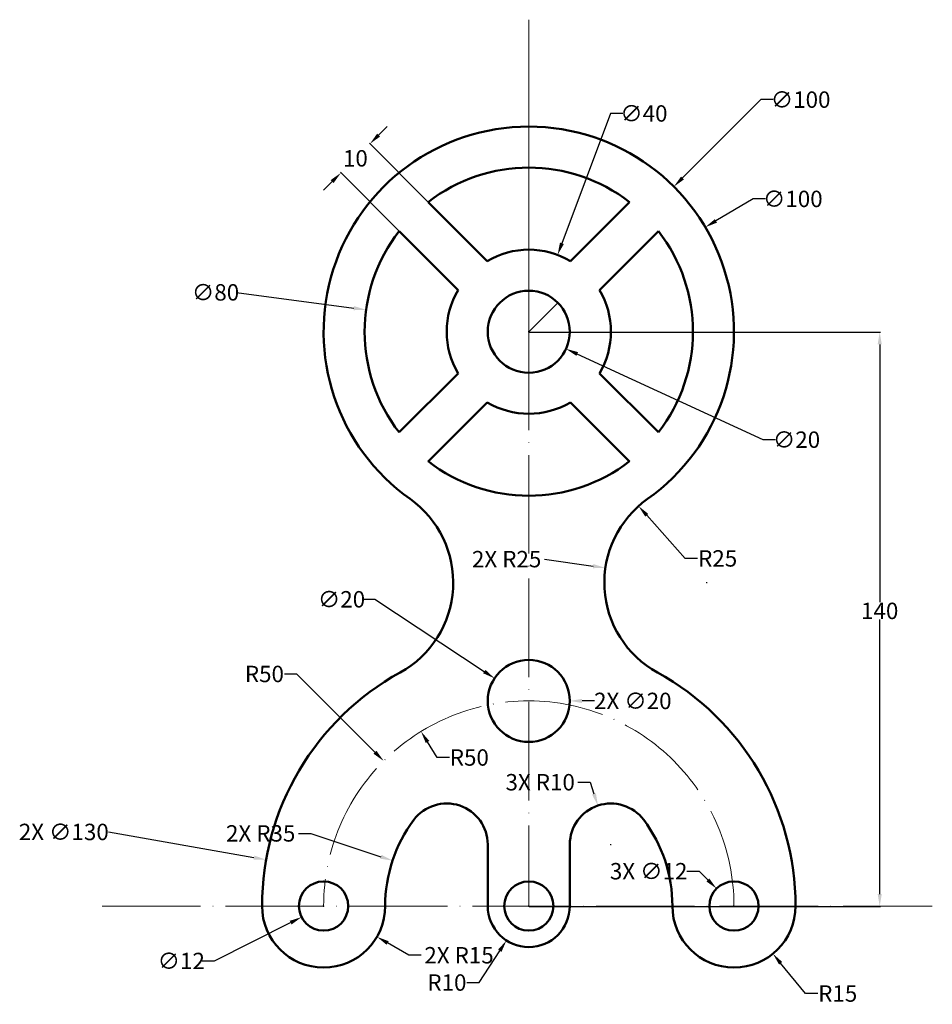
# Model space of a CAD drawing. Units: inches. Extents: x 540 to 763, y 295 to 535.
import ezdxf

# ---------------------------------------------------------------- set-up
doc = ezdxf.new("R2010")
doc.units = ezdxf.units.IN
doc.header["$MEASUREMENT"] = 0
doc.linetypes.add('ACAD_ISO04W100', pattern=[30, 24, -3, 0, -3])
for name, color, linetype, lineweight in [('M-CNTR', 4, 'ACAD_ISO04W100', 18), ('M-CONS', 8, 'Continuous', 13), ('M-DIMS', 2, 'Continuous', 25), ('M-OUTL', 7, 'Continuous', 50)]:
    doc.layers.add(name, color=color, linetype=linetype, lineweight=lineweight)
doc.styles.get("Standard").update_dxf_attribs({"font": 'arial.ttf'})
doc.dimstyles.get("Standard").update_dxf_attribs({"dimtxt": 4, "dimasz": 3, "dimexe": 0.18, "dimexo": 0.0625, "dimgap": 0.09, "dimtad": 0, "dimtih": 1, "dimtoh": 1, "dimdec": 0, "dimzin": 0, "dimdsep": 46, "dimtxsty": 'Standard', "dimcen": 0.09, "dimadec": 0, "dimazin": 0, "dimtfac": 1, "dimtdec": 0, "dimtofl": 0, "dimtmove": 0, "dimatfit": 3, "dimfxl": 1, "dimtolj": 1, "dimtzin": 0, "dimarcsym": 0})

# ---------------------------------------------------------------- blocks, each defined once
blk = doc.blocks.new('*U1')
for p, q in [((-10.72, -3.65), (3.65, 10.72)), ((-3.65, -10.72), (10.72, 3.65))]:
    blk.add_line(p, q)
blk = doc.blocks.new('*U2')
at = {"layer": 'M-OUTL', "color": 0, "linetype": 'ByBlock', "lineweight": -2, "transparency": 16777216}
for p, rotation in [((643.5, 480.1), 90.00000000000003), ((643.5, 438.34), 180), ((685.26, 438.34), 270.0000000000001)]:
    blk.add_blockref('*U1', p, dxfattribs=dict(at, rotation=rotation))
blk.add_blockref('*U1', (685.26, 480.1), dxfattribs=at)
blk = doc.blocks.new('*D3')
at = {"layer": 'Defpoints', "color": 0, "transparency": 16777216}
for p in [(625.66, 505.02), (639.85, 490.82), (632.78, 483.75)]:
    blk.add_point(p, dxfattribs=at)
at = {"layer": 'M-DIMS', "color": 0, "lineweight": -2, "transparency": 16777216}
for p, q in [((627.78, 507.14), (629.9, 509.26)), ((639.81, 490.86), (625.53, 505.14)), ((632.74, 483.79), (618.46, 498.07)), ((616.46, 495.82), (614.34, 493.7))]:
    blk.add_line(p, q, dxfattribs=at)
at = {"layer": 'M-DIMS', "color": 0, "transparency": 16777216}
for points in [[(627.42, 507.49), (628.13, 506.78), (625.66, 505.02)], [(616.11, 496.18), (616.82, 495.47), (618.59, 497.94)]]:
    blk.add_solid(points, dxfattribs=at)
at = {"layer": 'M-DIMS', "color": 0, "transparency": 16777216, "insert": (622.12, 501.48), "char_height": 4, "attachment_point": 5}
blk.add_mtext('\\A1;10', dxfattribs=at)
blk = doc.blocks.new('*D4')
at = {"layer": 'Defpoints', "color": 0, "transparency": 16777216}
for p in [(707.4, 484.7), (621.36, 433.74)]:
    blk.add_point(p, dxfattribs=at)
at = {"layer": 'M-DIMS', "color": 0, "lineweight": -2, "transparency": 16777216}
for p, q in [((719.05, 491.59), (709.98, 486.23)), ((722.05, 491.59), (719.05, 491.59)), ((664.29, 459.22), (664.47, 459.22)), ((664.38, 459.13), (664.38, 459.31))]:
    blk.add_line(p, q, dxfattribs=at)
at = {"layer": 'M-DIMS', "color": 0, "transparency": 16777216}
blk.add_solid([(709.73, 486.66), (710.24, 485.8), (707.4, 484.7)], dxfattribs=at)
at = {"layer": 'M-DIMS', "color": 0, "transparency": 16777216, "insert": (728.72, 491.59), "char_height": 4, "attachment_point": 5}
blk.add_mtext('\\A1;∅100', dxfattribs=at)
blk = doc.blocks.new('*D5')
at = {"layer": 'Defpoints', "color": 0, "transparency": 16777216}
for p in [(624.74, 464.56), (704.02, 453.88)]:
    blk.add_point(p, dxfattribs=at)
at = {"layer": 'M-DIMS', "color": 0, "lineweight": -2, "transparency": 16777216}
for p, q in [((593.17, 468.81), (621.76, 464.96)), ((664.29, 459.22), (664.47, 459.22)), ((664.38, 459.13), (664.38, 459.31))]:
    blk.add_line(p, q, dxfattribs=at)
at = {"layer": 'M-DIMS', "color": 0, "transparency": 16777216}
blk.add_solid([(621.83, 465.45), (621.7, 464.46), (624.74, 464.56)], dxfattribs=at)
at = {"layer": 'M-DIMS', "color": 0, "transparency": 16777216, "insert": (588.04, 468.81), "char_height": 4, "attachment_point": 5}
blk.add_mtext('\\A1;∅80', dxfattribs=at)
blk = doc.blocks.new('*D6')
at = {"layer": 'Defpoints', "color": 0, "transparency": 16777216}
for p in [(671.4, 477.95), (657.36, 440.49)]:
    blk.add_point(p, dxfattribs=at)
at = {"layer": 'M-DIMS', "color": 0, "lineweight": -2, "transparency": 16777216}
for p, q in [((684.31, 512.42), (672.45, 480.76)), ((687.31, 512.42), (684.31, 512.42)), ((664.29, 459.22), (664.47, 459.22)), ((664.38, 459.13), (664.38, 459.31))]:
    blk.add_line(p, q, dxfattribs=at)
at = {"layer": 'M-DIMS', "color": 0, "transparency": 16777216}
blk.add_solid([(671.98, 480.94), (672.92, 480.58), (671.4, 477.95)], dxfattribs=at)
at = {"layer": 'M-DIMS', "color": 0, "transparency": 16777216, "insert": (692.43, 512.42), "char_height": 4, "attachment_point": 5}
blk.add_mtext('\\A1;∅40', dxfattribs=at)
blk = doc.blocks.new('*D7')
at = {"layer": 'Defpoints', "color": 0, "transparency": 16777216}
for p in [(655.3, 463.41), (673.46, 455.04)]:
    blk.add_point(p, dxfattribs=at)
at = {"layer": 'M-DIMS', "color": 0, "lineweight": -2, "transparency": 16777216}
for p, q in [((664.29, 459.22), (664.47, 459.22)), ((664.38, 459.13), (664.38, 459.31)), ((721.51, 432.9), (676.19, 453.78)), ((724.51, 432.9), (721.51, 432.9))]:
    blk.add_line(p, q, dxfattribs=at)
at = {"layer": 'M-DIMS', "color": 0, "transparency": 16777216}
blk.add_solid([(676.4, 454.24), (675.98, 453.33), (673.46, 455.04)], dxfattribs=at)
at = {"layer": 'M-DIMS', "color": 0, "transparency": 16777216, "insert": (729.63, 432.9), "char_height": 4, "attachment_point": 5}
blk.add_mtext('\\A1;∅20', dxfattribs=at)
blk = doc.blocks.new('*D8')
at = {"layer": 'Defpoints', "color": 0, "transparency": 16777216}
for p in [(664.38, 319.22), (658.94, 310.83)]:
    blk.add_point(p, dxfattribs=at)
at = {"layer": 'M-DIMS', "color": 0, "lineweight": -2, "transparency": 16777216}
for p, q in [((664.29, 319.22), (664.47, 319.22)), ((664.38, 319.13), (664.38, 319.31)), ((652.29, 300.57), (657.31, 308.31)), ((649.29, 300.57), (652.29, 300.57))]:
    blk.add_line(p, q, dxfattribs=at)
at = {"layer": 'M-DIMS', "color": 0, "transparency": 16777216}
blk.add_solid([(656.89, 308.58), (657.73, 308.04), (658.94, 310.83)], dxfattribs=at)
at = {"layer": 'M-DIMS', "color": 0, "transparency": 16777216, "insert": (644.43, 300.57), "char_height": 4, "attachment_point": 5}
blk.add_mtext('\\A1;R10', dxfattribs=at)
blk = doc.blocks.new('*D9')
at = {"layer": 'Defpoints', "color": 0, "transparency": 16777216}
for p in [(619.74, 321.92), (609.02, 316.52)]:
    blk.add_point(p, dxfattribs=at)
at = {"layer": 'M-DIMS', "color": 0, "lineweight": -2, "transparency": 16777216}
for p, q in [((614.29, 319.22), (614.47, 319.22)), ((614.38, 319.13), (614.38, 319.31)), ((587.8, 305.83), (606.34, 315.17)), ((584.8, 305.83), (587.8, 305.83))]:
    blk.add_line(p, q, dxfattribs=at)
at = {"layer": 'M-DIMS', "color": 0, "transparency": 16777216}
blk.add_solid([(606.12, 315.62), (606.57, 314.73), (609.02, 316.52)], dxfattribs=at)
at = {"layer": 'M-DIMS', "color": 0, "transparency": 16777216, "insert": (579.68, 305.83), "char_height": 4, "attachment_point": 5}
blk.add_mtext('\\A1;∅12', dxfattribs=at)
blk = doc.blocks.new('*D10')
at = {"layer": 'Defpoints', "color": 0, "transparency": 16777216}
for p in [(714.38, 319.22), (723.86, 307.6)]:
    blk.add_point(p, dxfattribs=at)
at = {"layer": 'M-DIMS', "color": 0, "lineweight": -2, "transparency": 16777216}
for p, q in [((714.29, 319.22), (714.47, 319.22)), ((714.38, 319.13), (714.38, 319.31)), ((731.78, 297.89), (725.76, 305.27)), ((734.78, 297.89), (731.78, 297.89))]:
    blk.add_line(p, q, dxfattribs=at)
at = {"layer": 'M-DIMS', "color": 0, "transparency": 16777216}
blk.add_solid([(726.14, 305.59), (725.37, 304.96), (723.86, 307.6)], dxfattribs=at)
at = {"layer": 'M-DIMS', "color": 0, "transparency": 16777216, "insert": (739.67, 297.89), "char_height": 4, "attachment_point": 5}
blk.add_mtext('\\A1;R15', dxfattribs=at)
blk = doc.blocks.new('*D11')
at = {"layer": 'Defpoints', "color": 0, "transparency": 16777216}
for p in [(656.03, 374.73), (672.72, 363.71)]:
    blk.add_point(p, dxfattribs=at)
at = {"layer": 'M-DIMS', "color": 0, "lineweight": -2, "transparency": 16777216}
for p, q in [((623.86, 393.99), (626.86, 393.99)), ((626.86, 393.99), (653.53, 376.38)), ((664.29, 369.22), (664.47, 369.22)), ((664.38, 369.13), (664.38, 369.31))]:
    blk.add_line(p, q, dxfattribs=at)
at = {"layer": 'M-DIMS', "color": 0, "transparency": 16777216}
blk.add_solid([(653.81, 376.8), (653.25, 375.97), (656.03, 374.73)], dxfattribs=at)
at = {"layer": 'M-DIMS', "color": 0, "transparency": 16777216, "insert": (618.74, 393.99), "char_height": 4, "attachment_point": 5}
blk.add_mtext('\\A1;∅20', dxfattribs=at)
blk = doc.blocks.new('*D12')
at = {"layer": 'Defpoints', "color": 0, "transparency": 16777216}
for p in [(638.12, 361.77), (664.38, 319.22)]:
    blk.add_point(p, dxfattribs=at)
at = {"layer": 'M-DIMS', "color": 0, "lineweight": -2, "transparency": 16777216}
for p, q in [((642.03, 355.43), (639.69, 359.22)), ((645.03, 355.43), (642.03, 355.43))]:
    blk.add_line(p, q, dxfattribs=at)
at = {"layer": 'M-DIMS', "color": 0, "transparency": 16777216}
blk.add_solid([(640.12, 359.48), (639.27, 358.95), (638.12, 361.77)], dxfattribs=at)
at = {"layer": 'M-DIMS', "color": 0, "transparency": 16777216, "insert": (649.89, 355.43), "char_height": 4, "attachment_point": 5}
blk.add_mtext('\\A1;R50', dxfattribs=at)
blk = doc.blocks.new('*D13')
at = {"layer": 'Defpoints', "color": 0, "transparency": 16777216}
for p in [(691.13, 416.71), (707.79, 398.06)]:
    blk.add_point(p, dxfattribs=at)
at = {"layer": 'M-DIMS', "color": 0, "lineweight": -2, "transparency": 16777216}
for p, q in [((702.52, 403.96), (693.13, 414.47)), ((705.52, 403.96), (702.52, 403.96))]:
    blk.add_line(p, q, dxfattribs=at)
at = {"layer": 'M-DIMS', "color": 0, "transparency": 16777216}
blk.add_solid([(693.5, 414.8), (692.76, 414.13), (691.13, 416.71)], dxfattribs=at)
at = {"layer": 'M-DIMS', "color": 0, "transparency": 16777216, "insert": (710.41, 403.96), "char_height": 4, "attachment_point": 5}
blk.add_mtext('\\A1;R25', dxfattribs=at)
blk = doc.blocks.new('*D14')
at = {"layer": 'Defpoints', "color": 0, "transparency": 16777216}
for p in [(664.38, 459.13), (664.38, 319.13), (749.9, 319.13)]:
    blk.add_point(p, dxfattribs=at)
at = {"layer": 'M-DIMS', "color": 0, "lineweight": -2, "transparency": 16777216}
for p, q in [((664.44, 459.13), (750.08, 459.13)), ((749.9, 456.13), (749.9, 393.31)), ((749.9, 322.13), (749.9, 389.04)), ((664.44, 319.13), (750.08, 319.13))]:
    blk.add_line(p, q, dxfattribs=at)
at = {"layer": 'M-DIMS', "color": 0, "transparency": 16777216}
for points in [[(749.4, 456.13), (750.4, 456.13), (749.9, 459.13)], [(749.4, 322.13), (750.4, 322.13), (749.9, 319.13)]]:
    blk.add_solid(points, dxfattribs=at)
at = {"layer": 'M-DIMS', "color": 0, "transparency": 16777216, "insert": (749.9, 391.17), "char_height": 4, "attachment_point": 5}
blk.add_mtext('\\A1;140', dxfattribs=at)
blk = doc.blocks.new('MOUNT-HOLE-D12')
blk.add_circle((0, 0), 6)
blk = doc.blocks.new('BORE-D20')
blk.add_circle((0, 0), 10)
blk = doc.blocks.new('*D17')
at = {"layer": 'Defpoints', "color": 0, "transparency": 16777216}
for p in [(600.37, 330.51), (728.39, 307.93)]:
    blk.add_point(p, dxfattribs=at)
at = {"layer": 'M-DIMS', "color": 0, "lineweight": -2, "transparency": 16777216}
for p, q in [((561.96, 337.28), (597.41, 331.03)), ((664.29, 319.22), (664.47, 319.22)), ((664.38, 319.13), (664.38, 319.31))]:
    blk.add_line(p, q, dxfattribs=at)
at = {"layer": 'M-DIMS', "color": 0, "transparency": 16777216}
blk.add_solid([(597.5, 331.52), (597.33, 330.54), (600.37, 330.51)], dxfattribs=at)
at = {"layer": 'M-DIMS', "color": 0, "transparency": 16777216, "insert": (551.06, 337.28), "char_height": 4, "attachment_point": 5}
blk.add_mtext('\\A1;2X ∅130', dxfattribs=at)
blk = doc.blocks.new('*D18')
at = {"layer": 'Defpoints', "color": 0, "transparency": 16777216}
for p in [(631.18, 330.29), (664.38, 319.22)]:
    blk.add_point(p, dxfattribs=at)
at = {"layer": 'M-DIMS', "color": 0, "lineweight": -2, "transparency": 16777216}
for p, q in [((608.25, 336.93), (611.25, 336.93)), ((611.25, 336.93), (628.33, 331.24)), ((664.29, 319.22), (664.47, 319.22)), ((664.38, 319.13), (664.38, 319.31))]:
    blk.add_line(p, q, dxfattribs=at)
at = {"layer": 'M-DIMS', "color": 0, "transparency": 16777216}
blk.add_solid([(628.49, 331.71), (628.17, 330.76), (631.18, 330.29)], dxfattribs=at)
at = {"layer": 'M-DIMS', "color": 0, "transparency": 16777216, "insert": (599.04, 336.93), "char_height": 4, "attachment_point": 5}
blk.add_mtext('\\A1;2X R35', dxfattribs=at)
blk = doc.blocks.new('*D19')
at = {"layer": 'Defpoints', "color": 0, "transparency": 16777216}
for p in [(681.22, 343.71), (684.38, 334.22)]:
    blk.add_point(p, dxfattribs=at)
at = {"layer": 'M-DIMS', "color": 0, "lineweight": -2, "transparency": 16777216}
for p, q in [((676.32, 349.4), (679.32, 349.4)), ((679.32, 349.4), (680.27, 346.55)), ((684.29, 334.22), (684.47, 334.22)), ((684.38, 334.13), (684.38, 334.31))]:
    blk.add_line(p, q, dxfattribs=at)
at = {"layer": 'M-DIMS', "color": 0, "transparency": 16777216}
blk.add_solid([(680.74, 346.71), (679.79, 346.4), (681.22, 343.71)], dxfattribs=at)
at = {"layer": 'M-DIMS', "color": 0, "transparency": 16777216, "insert": (667.16, 349.4), "char_height": 4, "attachment_point": 5}
blk.add_mtext('\\A1;3X R10', dxfattribs=at)
blk = doc.blocks.new('*D20')
at = {"layer": 'Defpoints', "color": 0, "transparency": 16777216}
for p in [(654.38, 369.22), (674.38, 369.22)]:
    blk.add_point(p, dxfattribs=at)
at = {"layer": 'M-DIMS', "color": 0, "lineweight": -2, "transparency": 16777216}
for p, q in [((664.29, 369.22), (664.47, 369.22)), ((664.38, 369.13), (664.38, 369.31)), ((680.38, 369.22), (677.38, 369.22))]:
    blk.add_line(p, q, dxfattribs=at)
at = {"layer": 'M-DIMS', "color": 0, "transparency": 16777216}
blk.add_solid([(677.38, 369.72), (677.38, 368.72), (674.38, 369.22)], dxfattribs=at)
at = {"layer": 'M-DIMS', "color": 0, "transparency": 16777216, "insert": (689.73, 369.22), "char_height": 4, "attachment_point": 5}
blk.add_mtext('\\A1;2X ∅20', dxfattribs=at)
blk = doc.blocks.new('*D21')
at = {"layer": 'Defpoints', "color": 0, "transparency": 16777216}
for p in [(710.14, 323.46), (718.62, 314.98)]:
    blk.add_point(p, dxfattribs=at)
at = {"layer": 'M-DIMS', "color": 0, "lineweight": -2, "transparency": 16777216}
for p, q in [((702.89, 327.71), (705.89, 327.71)), ((705.89, 327.71), (708.02, 325.59)), ((714.29, 319.22), (714.47, 319.22)), ((714.38, 319.13), (714.38, 319.31))]:
    blk.add_line(p, q, dxfattribs=at)
at = {"layer": 'M-DIMS', "color": 0, "transparency": 16777216}
blk.add_solid([(708.37, 325.94), (707.66, 325.23), (710.14, 323.46)], dxfattribs=at)
at = {"layer": 'M-DIMS', "color": 0, "transparency": 16777216, "insert": (693.59, 327.71), "char_height": 4, "attachment_point": 5}
blk.add_mtext('\\A1;3X ∅12', dxfattribs=at)
blk = doc.blocks.new('*D22')
at = {"layer": 'Defpoints', "color": 0, "transparency": 16777216}
for p in [(699.73, 494.58), (629.02, 423.87)]:
    blk.add_point(p, dxfattribs=at)
at = {"layer": 'M-DIMS', "color": 0, "lineweight": -2, "transparency": 16777216}
for p, q in [((720.95, 515.79), (701.86, 496.7)), ((723.95, 515.79), (720.95, 515.79)), ((664.29, 459.22), (664.47, 459.22)), ((664.38, 459.13), (664.38, 459.31))]:
    blk.add_line(p, q, dxfattribs=at)
at = {"layer": 'M-DIMS', "color": 0, "transparency": 16777216}
blk.add_solid([(701.5, 497.05), (702.21, 496.35), (699.73, 494.58)], dxfattribs=at)
at = {"layer": 'M-DIMS', "color": 0, "transparency": 16777216, "insert": (730.63, 515.79), "char_height": 4, "attachment_point": 5}
blk.add_mtext('\\A1;∅100', dxfattribs=at)
blk = doc.blocks.new('*D23')
at = {"layer": 'Defpoints', "color": 0, "transparency": 16777216}
for p in [(683.05, 401.64), (707.79, 398.06)]:
    blk.add_point(p, dxfattribs=at)
at = {"layer": 'M-DIMS', "color": 0, "lineweight": -2, "transparency": 16777216}
for p, q in [((668.2, 403.78), (680.08, 402.06)), ((707.7, 398.06), (707.88, 398.06)), ((707.79, 397.97), (707.79, 398.15))]:
    blk.add_line(p, q, dxfattribs=at)
at = {"layer": 'M-DIMS', "color": 0, "transparency": 16777216}
blk.add_solid([(680.15, 402.56), (680, 401.57), (683.05, 401.64)], dxfattribs=at)
at = {"layer": 'M-DIMS', "color": 0, "transparency": 16777216, "insert": (658.98, 403.78), "char_height": 4, "attachment_point": 5}
blk.add_mtext('\\A1;2X R25', dxfattribs=at)
blk = doc.blocks.new('*D24')
at = {"layer": 'Defpoints', "color": 0, "transparency": 16777216}
for p in [(614.38, 319.22), (627.37, 311.72)]:
    blk.add_point(p, dxfattribs=at)
at = {"layer": 'M-DIMS', "color": 0, "lineweight": -2, "transparency": 16777216}
for p, q in [((614.29, 319.22), (614.47, 319.22)), ((614.38, 319.13), (614.38, 319.31)), ((635.16, 307.22), (629.97, 310.22)), ((638.16, 307.22), (635.16, 307.22))]:
    blk.add_line(p, q, dxfattribs=at)
at = {"layer": 'M-DIMS', "color": 0, "transparency": 16777216}
blk.add_solid([(630.22, 310.65), (629.72, 309.79), (627.37, 311.72)], dxfattribs=at)
at = {"layer": 'M-DIMS', "color": 0, "transparency": 16777216, "insert": (647.38, 307.22), "char_height": 4, "attachment_point": 5}
blk.add_mtext('\\A1;2X R15', dxfattribs=at)
blk = doc.blocks.new('*D25')
at = {"layer": 'Defpoints', "color": 0, "transparency": 16777216}
for p in [(629.02, 354.58), (664.38, 319.22)]:
    blk.add_point(p, dxfattribs=at)
at = {"layer": 'M-DIMS', "color": 0, "lineweight": -2, "transparency": 16777216}
for p, q in [((604.81, 375.79), (607.81, 375.79)), ((607.81, 375.79), (626.9, 356.7)), ((664.29, 319.22), (664.47, 319.22)), ((664.38, 319.13), (664.38, 319.31))]:
    blk.add_line(p, q, dxfattribs=at)
at = {"layer": 'M-DIMS', "color": 0, "transparency": 16777216}
blk.add_solid([(627.26, 357.05), (626.55, 356.34), (629.02, 354.58)], dxfattribs=at)
at = {"layer": 'M-DIMS', "color": 0, "transparency": 16777216, "insert": (599.95, 375.79), "char_height": 4, "attachment_point": 5}
blk.add_mtext('\\A1;R50', dxfattribs=at)

msp = doc.modelspace()

# ---------------------------------------------------------------- linework, layer by layer
at = {"layer": 'M-CNTR'}
for p, q in [((664.38, 459.22), (664.38, 319.22)), ((560.39, 319.22), (762.72, 319.22))]:
    msp.add_line(p, q, dxfattribs=at)
msp.add_arc((664.38, 319.22), 50, 0, 180, dxfattribs=at)
at = {"layer": 'M-CONS'}
for q in [(664.38, 535.28), (671.45, 466.29)]:
    msp.add_line((664.38, 459.22), q, dxfattribs=at)
at = {"layer": 'M-OUTL'}
for p, q in [((654.38, 319.22), (654.38, 334.22)), ((674.38, 319.22), (674.38, 334.22))]:
    msp.add_line(p, q, dxfattribs=at)
for centre, radius, start, end in [((664.38, 459.22), 50, 305.3655, 234.6345), ((664.38, 459.22), 40, 52.1808, 127.8192), ((664.38, 459.22), 40, 52.1808, 127.8192), ((664.38, 459.22), 40, 142.1808, 217.8192), ((664.38, 459.22), 40, 142.1808, 217.8192), ((664.38, 459.22), 40, 322.1808, 37.8192), ((664.38, 459.22), 40, 322.1808, 37.8192), ((664.38, 459.22), 20, 59.4775, 120.5225), ((664.38, 459.22), 20, 149.4775, 210.5225), ((664.38, 459.22), 20, 329.4775, 30.5225), ((664.38, 459.22), 20, 239.4775, 300.5225), ((664.38, 459.22), 40, 232.1808, 307.8192), ((664.38, 459.22), 40, 232.1808, 307.8192), ((620.97, 398.06), 25, 298.8374, 54.6345), ((707.79, 398.06), 25, 125.3655, 241.1626), ((664.38, 319.22), 65, 118.8374, 180), ((664.38, 319.22), 65, 0, 61.1626), ((644.38, 334.22), 10, 0, 143.1301), ((684.38, 334.22), 10, 36.8699, 180), ((664.38, 319.22), 35, 143.1301, 180), ((664.38, 319.22), 35, 0, 36.8699), ((614.38, 319.22), 15, 180, 0), ((664.38, 319.22), 10, 180, 0), ((714.38, 319.22), 15, 180, 0)]:
    msp.add_arc(centre, radius, start, end, dxfattribs=at)

# ---------------------------------------------------------------- block references
for name, p in [('*U2', (0, 0)), ('BORE-D20', (664.38, 459.22)), ('BORE-D20', (664.38, 369.22)), ('MOUNT-HOLE-D12', (614.38, 319.22)), ('MOUNT-HOLE-D12', (664.38, 319.22)), ('MOUNT-HOLE-D12', (714.38, 319.22))]:
    msp.add_blockref(name, p, dxfattribs=at)

# ---------------------------------------------------------------- dimensions: what is measured, and where the dimension line sits
at = {"layer": 'M-DIMS'}
for p1, p2, override, picture, middle in [((629.02, 423.87), (699.73, 494.58), {"dimdec": 0, "dimlfac": 1, "dimrnd": 0, "dimzin": 0, "dimdsep": 46, "dimlunit": 2}, '*D22', (730.63, 515.79)), ((657.36, 440.49), (671.4, 477.95), {"dimclrd": 0, "dimclre": 0, "dimclrt": 0}, '*D6', (692.43, 512.42)), ((621.36, 433.74), (707.4, 484.7), {"dimclrd": 0, "dimclre": 0, "dimclrt": 0}, '*D4', (728.72, 491.59)), ((704.02, 453.88), (624.74, 464.56), {"dimclrd": 0, "dimclre": 0, "dimclrt": 0}, '*D5', (593.17, 468.81)), ((655.3, 463.41), (673.46, 455.04), {"dimclrd": 0, "dimclre": 0, "dimclrt": 0}, '*D7', (729.63, 432.9)), ((672.72, 363.71), (656.03, 374.73), {"dimclrd": 0, "dimclre": 0, "dimclrt": 0}, '*D11', (618.74, 393.99)), ((619.74, 321.92), (609.02, 316.52), {"dimclrd": 0, "dimclre": 0, "dimclrt": 0}, '*D9', (579.68, 305.83))]:
    dim = msp.add_diameter_dim_2p(p1=p1, p2=p2, dimstyle='Standard', override=override, dxfattribs=at)
    dim.commit()
    dim.dimension.update_dxf_attribs({"geometry": picture, "text_midpoint": middle, "dimtype": 163})
dim = msp.add_linear_dim(base=(625.66, 505.02), p1=(632.78, 483.75), p2=(639.85, 490.82), angle=225, dimstyle='Standard', override={"dimclrd": 0, "dimclre": 0, "dimclrt": 0}, dxfattribs=at)
dim.commit()
dim.dimension.update_dxf_attribs({"geometry": '*D3', "text_midpoint": (622.12, 501.48)})
dim = msp.add_linear_dim(base=(749.9, 319.13), p1=(664.38, 459.13), p2=(664.38, 319.13), angle=90, dimstyle='Standard', override={"dimclrd": 0, "dimclre": 0, "dimclrt": 0}, dxfattribs=at)
dim.commit()
dim.dimension.update_dxf_attribs({"geometry": '*D14', "text_midpoint": (749.9, 391.17), "dimtype": 160})
for center, mpoint, override, picture, middle in [((707.79, 398.06), (691.13, 416.71), {"dimclrd": 0, "dimclre": 0, "dimclrt": 0}, '*D13', (710.41, 403.96)), ((664.38, 319.22), (629.02, 354.58), {"dimdec": 0, "dimlfac": 1, "dimrnd": 0, "dimzin": 0, "dimdsep": 46, "dimlunit": 2}, '*D25', (599.95, 375.79)), ((664.38, 319.22), (638.12, 361.77), {"dimclrd": 0, "dimclre": 0, "dimclrt": 0}, '*D12', (649.89, 355.43)), ((664.38, 319.22), (658.94, 310.83), {"dimclrd": 0, "dimclre": 0, "dimclrt": 0}, '*D8', (644.43, 300.57)), ((714.38, 319.22), (723.86, 307.6), {"dimclrd": 0, "dimclre": 0, "dimclrt": 0}, '*D10', (739.67, 297.89))]:
    dim = msp.add_radius_dim(center=center, mpoint=mpoint, dimstyle='Standard', override=override, dxfattribs=at)
    dim.commit()
    dim.dimension.update_dxf_attribs({"geometry": picture, "text_midpoint": middle, "dimtype": 164})
for center, mpoint, text, picture, middle in [((707.79, 398.06), (683.05, 401.64), '2X <>', '*D23', (668.2, 403.78)), ((684.38, 334.22), (681.22, 343.71), '3X <>', '*D19', (667.16, 349.4)), ((664.38, 319.22), (631.18, 330.29), '2X <>', '*D18', (599.04, 336.93)), ((614.38, 319.22), (627.37, 311.72), '2X <>', '*D24', (647.38, 307.22))]:
    dim = msp.add_radius_dim(center=center, mpoint=mpoint, text=text, dimstyle='Standard', override={"dimdec": 0, "dimlfac": 1, "dimrnd": 0, "dimzin": 0, "dimdsep": 46, "dimlunit": 2}, dxfattribs=at)
    dim.commit()
    dim.dimension.update_dxf_attribs({"geometry": picture, "text_midpoint": middle, "dimtype": 164})
for p1, p2, text, picture, middle in [((654.38, 369.22), (674.38, 369.22), '2X <>', '*D20', (680.38, 369.22)), ((728.39, 307.93), (600.37, 330.51), '2X <>', '*D17', (561.96, 337.28)), ((718.62, 314.98), (710.14, 323.46), '3X <>', '*D21', (693.59, 327.71))]:
    dim = msp.add_diameter_dim_2p(p1=p1, p2=p2, text=text, dimstyle='Standard', override={"dimdec": 0, "dimlfac": 1, "dimrnd": 0, "dimzin": 0, "dimdsep": 46, "dimlunit": 2}, dxfattribs=at)
    dim.commit()
    dim.dimension.update_dxf_attribs({"geometry": picture, "text_midpoint": middle, "dimtype": 163})

doc.saveas('drawing.dxf')
